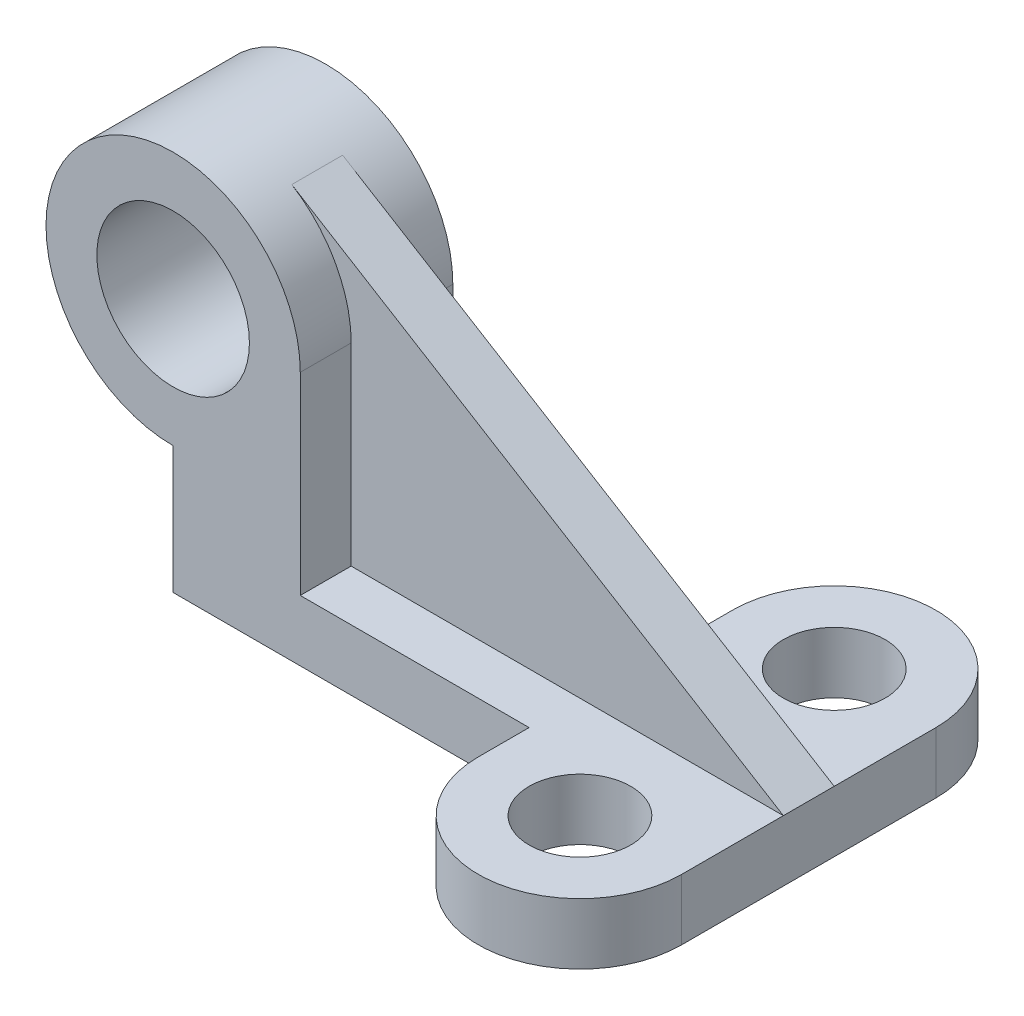
ISO-10303-21;
HEADER;
FILE_DESCRIPTION(('STEP AP214'),'2;1');
FILE_NAME('part.step','',(''),(''),'','','');
FILE_SCHEMA(('AUTOMOTIVE_DESIGN { 1 0 10303 214 1 1 1 1 }'));
ENDSEC;
DATA;
#1=APPLICATION_CONTEXT('core data for automotive mechanical design processes');
#2=APPLICATION_PROTOCOL_DEFINITION('international standard','automotive_design',2000,#1);
#3=PRODUCT_CONTEXT('',#1,'mechanical');
#4=PRODUCT('Part','Part','',(#3));
#5=PRODUCT_RELATED_PRODUCT_CATEGORY('part','',(#4));
#6=PRODUCT_DEFINITION_FORMATION('','',#4);
#7=PRODUCT_DEFINITION_CONTEXT('part definition',#1,'design');
#8=PRODUCT_DEFINITION('design','',#6,#7);
#9=PRODUCT_DEFINITION_SHAPE('','',#8);
#10=(LENGTH_UNIT() NAMED_UNIT(*) SI_UNIT(.MILLI.,.METRE.));
#11=(NAMED_UNIT(*) PLANE_ANGLE_UNIT() SI_UNIT($,.RADIAN.));
#12=(NAMED_UNIT(*) SI_UNIT($,.STERADIAN.) SOLID_ANGLE_UNIT());
#13=UNCERTAINTY_MEASURE_WITH_UNIT(LENGTH_MEASURE(1.E-05),#10,'distance_accuracy_value','');
#14=(GEOMETRIC_REPRESENTATION_CONTEXT(3) GLOBAL_UNCERTAINTY_ASSIGNED_CONTEXT((#13)) GLOBAL_UNIT_ASSIGNED_CONTEXT((#10,
#11,#12)) REPRESENTATION_CONTEXT('',''));
#15=CARTESIAN_POINT('',(0.,0.,0.));
#16=DIRECTION('',(0.,0.,1.));
#17=DIRECTION('',(1.,0.,0.));
#18=AXIS2_PLACEMENT_3D('',#15,#16,#17);
#19=CARTESIAN_POINT('',(0.,0.,0.));
#20=DIRECTION('',(0.,0.,1.));
#21=DIRECTION('',(1.,0.,0.));
#22=AXIS2_PLACEMENT_3D('',#19,#20,#21);
#23=PLANE('',#22);
#24=CARTESIAN_POINT('',(0.,0.,0.));
#25=DIRECTION('',(0.,0.,1.));
#26=DIRECTION('',(1.,0.,0.));
#27=AXIS2_PLACEMENT_3D('',#24,#25,#26);
#28=CIRCLE('',#27,15.);
#29=CARTESIAN_POINT('',(15.,0.,0.));
#30=VERTEX_POINT('',#29);
#31=EDGE_CURVE('E293',#30,#30,#28,.T.);
#32=ORIENTED_EDGE('',*,*,#31,.T.);
#33=EDGE_LOOP('',(#32));
#34=FACE_BOUND('',#33,.T.);
#35=DIRECTION('',(0.,1.,0.));
#36=VECTOR('',#35,1.);
#37=CARTESIAN_POINT('',(70.,-50.,0.));
#38=LINE('',#37,#36);
#39=CARTESIAN_POINT('',(70.,-50.,0.));
#40=VERTEX_POINT('',#39);
#41=CARTESIAN_POINT('',(70.,-38.,0.));
#42=VERTEX_POINT('',#41);
#43=EDGE_CURVE('E59',#40,#42,#38,.T.);
#44=ORIENTED_EDGE('',*,*,#43,.F.);
#45=DIRECTION('',(1.,0.,0.));
#46=VECTOR('',#45,1.);
#47=CARTESIAN_POINT('',(0.,-50.,0.));
#48=LINE('',#47,#46);
#49=CARTESIAN_POINT('',(0.,-50.,0.));
#50=VERTEX_POINT('',#49);
#51=EDGE_CURVE('E343',#50,#40,#48,.T.);
#52=ORIENTED_EDGE('',*,*,#51,.F.);
#53=DIRECTION('',(0.,-1.,0.));
#54=VECTOR('',#53,1.);
#55=CARTESIAN_POINT('',(0.,-25.,0.));
#56=LINE('',#55,#54);
#57=CARTESIAN_POINT('',(0.,-25.,0.));
#58=VERTEX_POINT('',#57);
#59=EDGE_CURVE('E352',#58,#50,#56,.T.);
#60=ORIENTED_EDGE('',*,*,#59,.F.);
#61=CARTESIAN_POINT('',(0.,0.,0.));
#62=DIRECTION('',(0.,0.,1.));
#63=DIRECTION('',(1.,0.,0.));
#64=AXIS2_PLACEMENT_3D('',#61,#62,#63);
#65=CIRCLE('',#64,25.);
#66=CARTESIAN_POINT('',(25.,0.,0.));
#67=VERTEX_POINT('',#66);
#68=EDGE_CURVE('E49',#67,#58,#65,.T.);
#69=ORIENTED_EDGE('',*,*,#68,.F.);
#70=DIRECTION('',(0.,1.,0.));
#71=VECTOR('',#70,1.);
#72=CARTESIAN_POINT('',(25.,-38.,0.));
#73=LINE('',#72,#71);
#74=CARTESIAN_POINT('',(25.,-38.,0.));
#75=VERTEX_POINT('',#74);
#76=EDGE_CURVE('E333',#75,#67,#73,.T.);
#77=ORIENTED_EDGE('',*,*,#76,.F.);
#78=DIRECTION('',(-1.,0.,0.));
#79=VECTOR('',#78,1.);
#80=CARTESIAN_POINT('',(80.,-38.,0.));
#81=LINE('',#80,#79);
#82=EDGE_CURVE('E340',#42,#75,#81,.T.);
#83=ORIENTED_EDGE('',*,*,#82,.F.);
#84=EDGE_LOOP('',(#44,#52,#60,#69,#77,#83));
#85=FACE_BOUND('',#84,.T.);
#86=ADVANCED_FACE('F39',(#34,#85),#23,.F.);
#87=CARTESIAN_POINT('',(0.,0.,30.));
#88=DIRECTION('',(0.,0.,1.));
#89=DIRECTION('',(1.,0.,0.));
#90=AXIS2_PLACEMENT_3D('',#87,#88,#89);
#91=PLANE('',#90);
#92=CARTESIAN_POINT('',(0.,0.,30.));
#93=DIRECTION('',(0.,0.,1.));
#94=DIRECTION('',(1.,0.,0.));
#95=AXIS2_PLACEMENT_3D('',#92,#93,#94);
#96=CIRCLE('',#95,15.);
#97=CARTESIAN_POINT('',(15.,0.,30.));
#98=VERTEX_POINT('',#97);
#99=EDGE_CURVE('E298',#98,#98,#96,.T.);
#100=ORIENTED_EDGE('',*,*,#99,.F.);
#101=EDGE_LOOP('',(#100));
#102=FACE_BOUND('',#101,.T.);
#103=DIRECTION('',(1.,0.,0.));
#104=VECTOR('',#103,1.);
#105=CARTESIAN_POINT('',(0.,-50.,30.));
#106=LINE('',#105,#104);
#107=CARTESIAN_POINT('',(0.,-50.,30.));
#108=VERTEX_POINT('',#107);
#109=CARTESIAN_POINT('',(70.,-50.,30.));
#110=VERTEX_POINT('',#109);
#111=EDGE_CURVE('E346',#108,#110,#106,.T.);
#112=ORIENTED_EDGE('',*,*,#111,.T.);
#113=DIRECTION('',(0.,1.,0.));
#114=VECTOR('',#113,1.);
#115=CARTESIAN_POINT('',(70.,-50.,30.));
#116=LINE('',#115,#114);
#117=CARTESIAN_POINT('',(70.,-38.,30.));
#118=VERTEX_POINT('',#117);
#119=EDGE_CURVE('E196',#110,#118,#116,.T.);
#120=ORIENTED_EDGE('',*,*,#119,.T.);
#121=DIRECTION('',(-1.,0.,0.));
#122=VECTOR('',#121,1.);
#123=CARTESIAN_POINT('',(80.,-38.,30.));
#124=LINE('',#123,#122);
#125=CARTESIAN_POINT('',(25.,-38.,30.));
#126=VERTEX_POINT('',#125);
#127=EDGE_CURVE('E353',#118,#126,#124,.T.);
#128=ORIENTED_EDGE('',*,*,#127,.T.);
#129=DIRECTION('',(0.,1.,0.));
#130=VECTOR('',#129,1.);
#131=CARTESIAN_POINT('',(25.,-38.,30.));
#132=LINE('',#131,#130);
#133=CARTESIAN_POINT('',(25.,0.,30.));
#134=VERTEX_POINT('',#133);
#135=EDGE_CURVE('E324',#126,#134,#132,.T.);
#136=ORIENTED_EDGE('',*,*,#135,.T.);
#137=CARTESIAN_POINT('',(0.,0.,30.));
#138=DIRECTION('',(0.,0.,1.));
#139=DIRECTION('',(1.,0.,0.));
#140=AXIS2_PLACEMENT_3D('',#137,#138,#139);
#141=CIRCLE('',#140,25.);
#142=CARTESIAN_POINT('',(0.,-25.,30.));
#143=VERTEX_POINT('',#142);
#144=EDGE_CURVE('E11',#134,#143,#141,.T.);
#145=ORIENTED_EDGE('',*,*,#144,.T.);
#146=DIRECTION('',(0.,-1.,0.));
#147=VECTOR('',#146,1.);
#148=CARTESIAN_POINT('',(0.,-25.,30.));
#149=LINE('',#148,#147);
#150=EDGE_CURVE('E344',#143,#108,#149,.T.);
#151=ORIENTED_EDGE('',*,*,#150,.T.);
#152=EDGE_LOOP('',(#112,#120,#128,#136,#145,#151));
#153=FACE_BOUND('',#152,.T.);
#154=ADVANCED_FACE('F282',(#102,#153),#91,.T.);
#155=CARTESIAN_POINT('',(0.,0.,30.));
#156=DIRECTION('',(0.,0.,-1.));
#157=DIRECTION('',(-1.,0.,0.));
#158=AXIS2_PLACEMENT_3D('',#155,#156,#157);
#159=CYLINDRICAL_SURFACE('',#158,25.);
#160=CARTESIAN_POINT('',(13.33493929526,21.1466166086145,20.));
#161=CARTESIAN_POINT('',(18.7792232306046,17.713481316683,20.));
#162=CARTESIAN_POINT('',(21.890334423913,12.0753160956246,20.));
#163=CARTESIAN_POINT('',(25.,6.43977071944921,20.));
#164=CARTESIAN_POINT('',(25.,0.,20.));
#165=B_SPLINE_CURVE_WITH_KNOTS('',2,(#160,#161,#162,#163,#164),.UNSPECIFIED.,.F.,.F.,(3,2,3),
(0.,0.5,1.),.UNSPECIFIED.);
#166=CARTESIAN_POINT('',(13.3325159789368,21.1428810416085,20.));
#167=VERTEX_POINT('',#166);
#168=CARTESIAN_POINT('',(25.,0.,20.));
#169=VERTEX_POINT('',#168);
#170=EDGE_CURVE('E158',#167,#169,#165,.T.);
#171=ORIENTED_EDGE('',*,*,#170,.F.);
#172=DIRECTION('',(0.,0.,-1.));
#173=VECTOR('',#172,1.);
#174=CARTESIAN_POINT('',(13.3349392952599,21.1466166086146,30.));
#175=LINE('',#174,#173);
#176=CARTESIAN_POINT('',(13.333271356551,21.1440454639604,10.));
#177=VERTEX_POINT('',#176);
#178=EDGE_CURVE('E217',#177,#167,#175,.F.);
#179=ORIENTED_EDGE('',*,*,#178,.F.);
#180=CARTESIAN_POINT('',(0.,0.,10.));
#181=DIRECTION('',(0.,0.,-1.));
#182=DIRECTION('',(0.5333975718104,0.84586466434458,0.));
#183=AXIS2_PLACEMENT_3D('',#180,#181,#182);
#184=CIRCLE('',#183,25.);
#185=CARTESIAN_POINT('',(25.,0.,10.));
#186=VERTEX_POINT('',#185);
#187=EDGE_CURVE('E225',#177,#186,#184,.T.);
#188=ORIENTED_EDGE('',*,*,#187,.T.);
#189=DIRECTION('',(0.,0.,1.));
#190=VECTOR('',#189,1.);
#191=CARTESIAN_POINT('',(25.,0.,0.));
#192=LINE('',#191,#190);
#193=EDGE_CURVE('E303',#67,#186,#192,.T.);
#194=ORIENTED_EDGE('',*,*,#193,.F.);
#195=ORIENTED_EDGE('',*,*,#68,.T.);
#196=DIRECTION('',(0.,0.,1.));
#197=VECTOR('',#196,1.);
#198=CARTESIAN_POINT('',(0.,-25.,0.));
#199=LINE('',#198,#197);
#200=EDGE_CURVE('E302',#58,#143,#199,.T.);
#201=ORIENTED_EDGE('',*,*,#200,.T.);
#202=ORIENTED_EDGE('',*,*,#144,.F.);
#203=EDGE_CURVE('E42',#169,#134,#192,.T.);
#204=ORIENTED_EDGE('',*,*,#203,.F.);
#205=EDGE_LOOP('',(#171,#179,#188,#194,#195,#201,#202,#204));
#206=FACE_BOUND('',#205,.T.);
#207=ADVANCED_FACE('F41',(#206),#159,.T.);
#208=CARTESIAN_POINT('',(25.,-38.,0.));
#209=DIRECTION('',(1.,0.,0.));
#210=DIRECTION('',(0.,0.,-1.));
#211=AXIS2_PLACEMENT_3D('',#208,#209,#210);
#212=PLANE('',#211);
#213=DIRECTION('',(0.,0.,1.));
#214=VECTOR('',#213,1.);
#215=CARTESIAN_POINT('',(25.,-38.,0.));
#216=LINE('',#215,#214);
#217=CARTESIAN_POINT('',(25.,-38.,20.));
#218=VERTEX_POINT('',#217);
#219=EDGE_CURVE('E329',#218,#126,#216,.T.);
#220=ORIENTED_EDGE('',*,*,#219,.F.);
#221=DIRECTION('',(0.,-1.,0.));
#222=VECTOR('',#221,1.);
#223=CARTESIAN_POINT('',(25.,0.,20.));
#224=LINE('',#223,#222);
#225=EDGE_CURVE('E211',#169,#218,#224,.T.);
#226=ORIENTED_EDGE('',*,*,#225,.F.);
#227=ORIENTED_EDGE('',*,*,#203,.T.);
#228=ORIENTED_EDGE('',*,*,#135,.F.);
#229=EDGE_LOOP('',(#220,#226,#227,#228));
#230=FACE_BOUND('',#229,.T.);
#231=ADVANCED_FACE('F271',(#230),#212,.T.);
#232=CARTESIAN_POINT('',(80.,-38.,0.));
#233=DIRECTION('',(0.,1.,0.));
#234=DIRECTION('',(-1.,0.,0.));
#235=AXIS2_PLACEMENT_3D('',#232,#233,#234);
#236=PLANE('',#235);
#237=CARTESIAN_POINT('',(90.,-38.,40.));
#238=DIRECTION('',(0.,1.,0.));
#239=DIRECTION('',(-1.,0.,0.));
#240=AXIS2_PLACEMENT_3D('',#237,#238,#239);
#241=CIRCLE('',#240,9.99999999999999);
#242=CARTESIAN_POINT('',(80.,-38.,40.));
#243=VERTEX_POINT('',#242);
#244=EDGE_CURVE('E183',#243,#243,#241,.T.);
#245=ORIENTED_EDGE('',*,*,#244,.F.);
#246=EDGE_LOOP('',(#245));
#247=FACE_BOUND('',#246,.T.);
#248=DIRECTION('',(0.,0.,1.));
#249=VECTOR('',#248,1.);
#250=CARTESIAN_POINT('',(110.,-38.,0.));
#251=LINE('',#250,#249);
#252=CARTESIAN_POINT('',(110.,-38.,20.));
#253=VERTEX_POINT('',#252);
#254=CARTESIAN_POINT('',(110.,-38.,40.));
#255=VERTEX_POINT('',#254);
#256=EDGE_CURVE('E160',#253,#255,#251,.T.);
#257=ORIENTED_EDGE('',*,*,#256,.F.);
#258=DIRECTION('',(1.,0.,0.));
#259=VECTOR('',#258,1.);
#260=CARTESIAN_POINT('',(25.,-38.,20.));
#261=LINE('',#260,#259);
#262=EDGE_CURVE('E210',#218,#253,#261,.T.);
#263=ORIENTED_EDGE('',*,*,#262,.F.);
#264=ORIENTED_EDGE('',*,*,#219,.T.);
#265=ORIENTED_EDGE('',*,*,#127,.F.);
#266=DIRECTION('',(0.,0.,1.));
#267=VECTOR('',#266,1.);
#268=CARTESIAN_POINT('',(70.,-38.,40.));
#269=LINE('',#268,#267);
#270=CARTESIAN_POINT('',(70.,-38.,40.));
#271=VERTEX_POINT('',#270);
#272=EDGE_CURVE('E68',#118,#271,#269,.T.);
#273=ORIENTED_EDGE('',*,*,#272,.T.);
#274=CARTESIAN_POINT('',(90.,-38.,40.));
#275=DIRECTION('',(0.,1.,0.));
#276=DIRECTION('',(1.,0.,0.));
#277=AXIS2_PLACEMENT_3D('',#274,#275,#276);
#278=CIRCLE('',#277,20.);
#279=EDGE_CURVE('E198',#271,#255,#278,.T.);
#280=ORIENTED_EDGE('',*,*,#279,.T.);
#281=EDGE_LOOP('',(#257,#263,#264,#265,#273,#280));
#282=FACE_BOUND('',#281,.T.);
#283=ADVANCED_FACE('F274',(#247,#282),#236,.T.);
#284=CARTESIAN_POINT('',(0.,0.,0.));
#285=DIRECTION('',(0.,0.,1.));
#286=DIRECTION('',(1.,0.,0.));
#287=AXIS2_PLACEMENT_3D('',#284,#285,#286);
#288=CYLINDRICAL_SURFACE('',#287,15.);
#289=ORIENTED_EDGE('',*,*,#31,.F.);
#290=EDGE_LOOP('',(#289));
#291=FACE_BOUND('',#290,.T.);
#292=ORIENTED_EDGE('',*,*,#99,.T.);
#293=EDGE_LOOP('',(#292));
#294=FACE_BOUND('',#293,.T.);
#295=ADVANCED_FACE('F267',(#291,#294),#288,.F.);
#296=DIRECTION('',(0.,-1.,0.));
#297=VECTOR('',#296,1.);
#298=CARTESIAN_POINT('',(25.,0.,10.));
#299=LINE('',#298,#297);
#300=CARTESIAN_POINT('',(25.,-38.,10.));
#301=VERTEX_POINT('',#300);
#302=EDGE_CURVE('E201',#186,#301,#299,.T.);
#303=ORIENTED_EDGE('',*,*,#302,.T.);
#304=EDGE_CURVE('E330',#75,#301,#216,.T.);
#305=ORIENTED_EDGE('',*,*,#304,.F.);
#306=ORIENTED_EDGE('',*,*,#76,.T.);
#307=ORIENTED_EDGE('',*,*,#193,.T.);
#308=EDGE_LOOP('',(#303,#305,#306,#307));
#309=FACE_BOUND('',#308,.T.);
#310=ADVANCED_FACE('F264',(#309),#212,.T.);
#311=CARTESIAN_POINT('',(90.,-38.,-10.));
#312=DIRECTION('',(0.,1.,0.));
#313=DIRECTION('',(-1.,0.,0.));
#314=AXIS2_PLACEMENT_3D('',#311,#312,#313);
#315=CIRCLE('',#314,9.99999999999999);
#316=CARTESIAN_POINT('',(80.,-38.,-10.));
#317=VERTEX_POINT('',#316);
#318=EDGE_CURVE('E177',#317,#317,#315,.T.);
#319=ORIENTED_EDGE('',*,*,#318,.F.);
#320=EDGE_LOOP('',(#319));
#321=FACE_BOUND('',#320,.T.);
#322=DIRECTION('',(1.,0.,0.));
#323=VECTOR('',#322,1.);
#324=CARTESIAN_POINT('',(25.,-38.,10.));
#325=LINE('',#324,#323);
#326=CARTESIAN_POINT('',(110.,-38.,10.));
#327=VERTEX_POINT('',#326);
#328=EDGE_CURVE('E215',#301,#327,#325,.T.);
#329=ORIENTED_EDGE('',*,*,#328,.T.);
#330=CARTESIAN_POINT('',(110.,-38.,-10.));
#331=VERTEX_POINT('',#330);
#332=EDGE_CURVE('E349',#331,#327,#251,.T.);
#333=ORIENTED_EDGE('',*,*,#332,.F.);
#334=CARTESIAN_POINT('',(90.,-38.,-10.));
#335=DIRECTION('',(0.,1.,0.));
#336=DIRECTION('',(-1.,0.,0.));
#337=AXIS2_PLACEMENT_3D('',#334,#335,#336);
#338=CIRCLE('',#337,20.);
#339=CARTESIAN_POINT('',(70.,-38.,-10.));
#340=VERTEX_POINT('',#339);
#341=EDGE_CURVE('E167',#331,#340,#338,.T.);
#342=ORIENTED_EDGE('',*,*,#341,.T.);
#343=DIRECTION('',(0.,0.,1.));
#344=VECTOR('',#343,1.);
#345=CARTESIAN_POINT('',(70.,-38.,-10.));
#346=LINE('',#345,#344);
#347=EDGE_CURVE('E171',#340,#42,#346,.T.);
#348=ORIENTED_EDGE('',*,*,#347,.T.);
#349=ORIENTED_EDGE('',*,*,#82,.T.);
#350=ORIENTED_EDGE('',*,*,#304,.T.);
#351=EDGE_LOOP('',(#329,#333,#342,#348,#349,#350));
#352=FACE_BOUND('',#351,.T.);
#353=ADVANCED_FACE('F268',(#321,#352),#236,.T.);
#354=CARTESIAN_POINT('',(0.,-50.,0.));
#355=DIRECTION('',(0.,-1.,0.));
#356=DIRECTION('',(0.,0.,-1.));
#357=AXIS2_PLACEMENT_3D('',#354,#355,#356);
#358=PLANE('',#357);
#359=CARTESIAN_POINT('',(90.,-50.,-10.));
#360=DIRECTION('',(0.,1.,0.));
#361=DIRECTION('',(-1.,0.,0.));
#362=AXIS2_PLACEMENT_3D('',#359,#360,#361);
#363=CIRCLE('',#362,9.99999999999999);
#364=CARTESIAN_POINT('',(80.,-50.,-10.));
#365=VERTEX_POINT('',#364);
#366=EDGE_CURVE('E185',#365,#365,#363,.T.);
#367=ORIENTED_EDGE('',*,*,#366,.T.);
#368=EDGE_LOOP('',(#367));
#369=FACE_BOUND('',#368,.T.);
#370=CARTESIAN_POINT('',(90.,-50.,40.));
#371=DIRECTION('',(0.,1.,0.));
#372=DIRECTION('',(-1.,0.,0.));
#373=AXIS2_PLACEMENT_3D('',#370,#371,#372);
#374=CIRCLE('',#373,9.99999999999999);
#375=CARTESIAN_POINT('',(80.,-50.,40.));
#376=VERTEX_POINT('',#375);
#377=EDGE_CURVE('E190',#376,#376,#374,.T.);
#378=ORIENTED_EDGE('',*,*,#377,.T.);
#379=EDGE_LOOP('',(#378));
#380=FACE_BOUND('',#379,.T.);
#381=ORIENTED_EDGE('',*,*,#111,.F.);
#382=DIRECTION('',(0.,0.,1.));
#383=VECTOR('',#382,1.);
#384=CARTESIAN_POINT('',(0.,-50.,0.));
#385=LINE('',#384,#383);
#386=EDGE_CURVE('E332',#50,#108,#385,.T.);
#387=ORIENTED_EDGE('',*,*,#386,.F.);
#388=ORIENTED_EDGE('',*,*,#51,.T.);
#389=DIRECTION('',(0.,0.,1.));
#390=VECTOR('',#389,1.);
#391=CARTESIAN_POINT('',(70.,-50.,-10.));
#392=LINE('',#391,#390);
#393=CARTESIAN_POINT('',(70.,-50.,-10.));
#394=VERTEX_POINT('',#393);
#395=EDGE_CURVE('E169',#394,#40,#392,.T.);
#396=ORIENTED_EDGE('',*,*,#395,.F.);
#397=CARTESIAN_POINT('',(90.,-50.,-10.));
#398=DIRECTION('',(0.,1.,0.));
#399=DIRECTION('',(-1.,0.,0.));
#400=AXIS2_PLACEMENT_3D('',#397,#398,#399);
#401=CIRCLE('',#400,20.);
#402=CARTESIAN_POINT('',(110.,-50.,-10.));
#403=VERTEX_POINT('',#402);
#404=EDGE_CURVE('E162',#403,#394,#401,.T.);
#405=ORIENTED_EDGE('',*,*,#404,.F.);
#406=DIRECTION('',(0.,0.,1.));
#407=VECTOR('',#406,1.);
#408=CARTESIAN_POINT('',(110.,-50.,0.));
#409=LINE('',#408,#407);
#410=CARTESIAN_POINT('',(110.,-50.,40.));
#411=VERTEX_POINT('',#410);
#412=EDGE_CURVE('E144',#403,#411,#409,.T.);
#413=ORIENTED_EDGE('',*,*,#412,.T.);
#414=CARTESIAN_POINT('',(90.,-50.,40.));
#415=DIRECTION('',(0.,1.,0.));
#416=DIRECTION('',(1.,0.,0.));
#417=AXIS2_PLACEMENT_3D('',#414,#415,#416);
#418=CIRCLE('',#417,20.);
#419=CARTESIAN_POINT('',(70.,-50.,40.));
#420=VERTEX_POINT('',#419);
#421=EDGE_CURVE('E194',#420,#411,#418,.T.);
#422=ORIENTED_EDGE('',*,*,#421,.F.);
#423=DIRECTION('',(0.,0.,1.));
#424=VECTOR('',#423,1.);
#425=CARTESIAN_POINT('',(70.,-50.,40.));
#426=LINE('',#425,#424);
#427=EDGE_CURVE('E195',#110,#420,#426,.T.);
#428=ORIENTED_EDGE('',*,*,#427,.F.);
#429=EDGE_LOOP('',(#381,#387,#388,#396,#405,#413,#422,#428));
#430=FACE_BOUND('',#429,.T.);
#431=ADVANCED_FACE('F173',(#369,#380,#430),#358,.T.);
#432=CARTESIAN_POINT('',(0.,-25.,0.));
#433=DIRECTION('',(-1.,0.,0.));
#434=DIRECTION('',(0.,-1.,0.));
#435=AXIS2_PLACEMENT_3D('',#432,#433,#434);
#436=PLANE('',#435);
#437=ORIENTED_EDGE('',*,*,#150,.F.);
#438=ORIENTED_EDGE('',*,*,#200,.F.);
#439=ORIENTED_EDGE('',*,*,#59,.T.);
#440=ORIENTED_EDGE('',*,*,#386,.T.);
#441=EDGE_LOOP('',(#437,#438,#439,#440));
#442=FACE_BOUND('',#441,.T.);
#443=ADVANCED_FACE('F262',(#442),#436,.T.);
#444=CARTESIAN_POINT('',(110.,-50.,0.));
#445=DIRECTION('',(1.,0.,0.));
#446=DIRECTION('',(0.,0.,-1.));
#447=AXIS2_PLACEMENT_3D('',#444,#445,#446);
#448=PLANE('',#447);
#449=ORIENTED_EDGE('',*,*,#256,.T.);
#450=DIRECTION('',(0.,1.,0.));
#451=VECTOR('',#450,1.);
#452=CARTESIAN_POINT('',(110.,-50.,40.));
#453=LINE('',#452,#451);
#454=EDGE_CURVE('E155',#411,#255,#453,.T.);
#455=ORIENTED_EDGE('',*,*,#454,.F.);
#456=ORIENTED_EDGE('',*,*,#412,.F.);
#457=DIRECTION('',(0.,1.,0.));
#458=VECTOR('',#457,1.);
#459=CARTESIAN_POINT('',(110.,-50.,-10.));
#460=LINE('',#459,#458);
#461=EDGE_CURVE('E149',#403,#331,#460,.T.);
#462=ORIENTED_EDGE('',*,*,#461,.T.);
#463=ORIENTED_EDGE('',*,*,#332,.T.);
#464=DIRECTION('',(0.,0.,-1.));
#465=VECTOR('',#464,1.);
#466=CARTESIAN_POINT('',(110.,-38.,20.));
#467=LINE('',#466,#465);
#468=EDGE_CURVE('E216',#253,#327,#467,.T.);
#469=ORIENTED_EDGE('',*,*,#468,.F.);
#470=EDGE_LOOP('',(#449,#455,#456,#462,#463,#469));
#471=FACE_BOUND('',#470,.T.);
#472=ADVANCED_FACE('F150',(#471),#448,.T.);
#473=CARTESIAN_POINT('',(-0.607605139838045,-0.345958865427095,20.));
#474=DIRECTION('',(0.,0.,-1.));
#475=DIRECTION('',(-1.,0.,0.));
#476=AXIS2_PLACEMENT_3D('',#473,#474,#475);
#477=PLANE('',#476);
#478=DIRECTION('',(-0.852993027350446,0.521922307715929,0.));
#479=VECTOR('',#478,1.);
#480=CARTESIAN_POINT('',(110.,-38.,20.));
#481=LINE('',#480,#479);
#482=EDGE_CURVE('E209',#253,#167,#481,.T.);
#483=ORIENTED_EDGE('',*,*,#482,.T.);
#484=ORIENTED_EDGE('',*,*,#170,.T.);
#485=ORIENTED_EDGE('',*,*,#225,.T.);
#486=ORIENTED_EDGE('',*,*,#262,.T.);
#487=EDGE_LOOP('',(#483,#484,#485,#486));
#488=FACE_BOUND('',#487,.T.);
#489=ADVANCED_FACE('F254',(#488),#477,.F.);
#490=CARTESIAN_POINT('',(-0.607605139838045,-0.345958865427095,10.));
#491=DIRECTION('',(0.,0.,-1.));
#492=DIRECTION('',(-1.,0.,0.));
#493=AXIS2_PLACEMENT_3D('',#490,#491,#492);
#494=PLANE('',#493);
#495=ORIENTED_EDGE('',*,*,#187,.F.);
#496=DIRECTION('',(-0.852993027350446,0.521922307715929,0.));
#497=VECTOR('',#496,1.);
#498=CARTESIAN_POINT('',(110.,-38.,10.));
#499=LINE('',#498,#497);
#500=EDGE_CURVE('E214',#327,#177,#499,.T.);
#501=ORIENTED_EDGE('',*,*,#500,.F.);
#502=ORIENTED_EDGE('',*,*,#328,.F.);
#503=ORIENTED_EDGE('',*,*,#302,.F.);
#504=EDGE_LOOP('',(#495,#501,#502,#503));
#505=FACE_BOUND('',#504,.T.);
#506=ADVANCED_FACE('F244',(#505),#494,.T.);
#507=CARTESIAN_POINT('',(110.,-38.,20.));
#508=DIRECTION('',(-0.521922307715929,-0.852993027350446,0.));
#509=DIRECTION('',(0.852993027350446,-0.521922307715929,0.));
#510=AXIS2_PLACEMENT_3D('',#507,#508,#509);
#511=PLANE('',#510);
#512=ORIENTED_EDGE('',*,*,#500,.T.);
#513=ORIENTED_EDGE('',*,*,#178,.T.);
#514=ORIENTED_EDGE('',*,*,#482,.F.);
#515=ORIENTED_EDGE('',*,*,#468,.T.);
#516=EDGE_LOOP('',(#512,#513,#514,#515));
#517=FACE_BOUND('',#516,.T.);
#518=ADVANCED_FACE('F255',(#517),#511,.F.);
#519=CARTESIAN_POINT('',(90.,-50.,40.));
#520=DIRECTION('',(0.,1.,0.));
#521=DIRECTION('',(-1.,0.,0.));
#522=AXIS2_PLACEMENT_3D('',#519,#520,#521);
#523=CYLINDRICAL_SURFACE('',#522,20.);
#524=ORIENTED_EDGE('',*,*,#279,.F.);
#525=DIRECTION('',(0.,1.,0.));
#526=VECTOR('',#525,1.);
#527=CARTESIAN_POINT('',(70.,-50.,40.));
#528=LINE('',#527,#526);
#529=EDGE_CURVE('E204',#420,#271,#528,.T.);
#530=ORIENTED_EDGE('',*,*,#529,.F.);
#531=ORIENTED_EDGE('',*,*,#421,.T.);
#532=ORIENTED_EDGE('',*,*,#454,.T.);
#533=EDGE_LOOP('',(#524,#530,#531,#532));
#534=FACE_BOUND('',#533,.T.);
#535=ADVANCED_FACE('F257',(#534),#523,.T.);
#536=CARTESIAN_POINT('',(70.,-50.,40.));
#537=DIRECTION('',(-1.,0.,0.));
#538=DIRECTION('',(0.,-1.,0.));
#539=AXIS2_PLACEMENT_3D('',#536,#537,#538);
#540=PLANE('',#539);
#541=ORIENTED_EDGE('',*,*,#272,.F.);
#542=ORIENTED_EDGE('',*,*,#119,.F.);
#543=ORIENTED_EDGE('',*,*,#427,.T.);
#544=ORIENTED_EDGE('',*,*,#529,.T.);
#545=EDGE_LOOP('',(#541,#542,#543,#544));
#546=FACE_BOUND('',#545,.T.);
#547=ADVANCED_FACE('F390',(#546),#540,.T.);
#548=CARTESIAN_POINT('',(90.,-50.,40.));
#549=DIRECTION('',(0.,1.,0.));
#550=DIRECTION('',(-1.,0.,0.));
#551=AXIS2_PLACEMENT_3D('',#548,#549,#550);
#552=CYLINDRICAL_SURFACE('',#551,9.99999999999999);
#553=ORIENTED_EDGE('',*,*,#377,.F.);
#554=EDGE_LOOP('',(#553));
#555=FACE_BOUND('',#554,.T.);
#556=ORIENTED_EDGE('',*,*,#244,.T.);
#557=EDGE_LOOP('',(#556));
#558=FACE_BOUND('',#557,.T.);
#559=ADVANCED_FACE('F386',(#555,#558),#552,.F.);
#560=CARTESIAN_POINT('',(70.,-50.,-10.));
#561=DIRECTION('',(-1.,0.,0.));
#562=DIRECTION('',(0.,0.,1.));
#563=AXIS2_PLACEMENT_3D('',#560,#561,#562);
#564=PLANE('',#563);
#565=ORIENTED_EDGE('',*,*,#347,.F.);
#566=DIRECTION('',(0.,1.,0.));
#567=VECTOR('',#566,1.);
#568=CARTESIAN_POINT('',(70.,-50.,-10.));
#569=LINE('',#568,#567);
#570=EDGE_CURVE('E170',#394,#340,#569,.T.);
#571=ORIENTED_EDGE('',*,*,#570,.F.);
#572=ORIENTED_EDGE('',*,*,#395,.T.);
#573=ORIENTED_EDGE('',*,*,#43,.T.);
#574=EDGE_LOOP('',(#565,#571,#572,#573));
#575=FACE_BOUND('',#574,.T.);
#576=ADVANCED_FACE('F379',(#575),#564,.T.);
#577=CARTESIAN_POINT('',(90.,-50.,-10.));
#578=DIRECTION('',(0.,1.,0.));
#579=DIRECTION('',(-1.,0.,0.));
#580=AXIS2_PLACEMENT_3D('',#577,#578,#579);
#581=CYLINDRICAL_SURFACE('',#580,20.);
#582=ORIENTED_EDGE('',*,*,#341,.F.);
#583=ORIENTED_EDGE('',*,*,#461,.F.);
#584=ORIENTED_EDGE('',*,*,#404,.T.);
#585=ORIENTED_EDGE('',*,*,#570,.T.);
#586=EDGE_LOOP('',(#582,#583,#584,#585));
#587=FACE_BOUND('',#586,.T.);
#588=ADVANCED_FACE('F165',(#587),#581,.T.);
#589=CARTESIAN_POINT('',(90.,-50.,-10.));
#590=DIRECTION('',(0.,1.,0.));
#591=DIRECTION('',(-1.,0.,0.));
#592=AXIS2_PLACEMENT_3D('',#589,#590,#591);
#593=CYLINDRICAL_SURFACE('',#592,9.99999999999999);
#594=ORIENTED_EDGE('',*,*,#366,.F.);
#595=EDGE_LOOP('',(#594));
#596=FACE_BOUND('',#595,.T.);
#597=ORIENTED_EDGE('',*,*,#318,.T.);
#598=EDGE_LOOP('',(#597));
#599=FACE_BOUND('',#598,.T.);
#600=ADVANCED_FACE('F399',(#596,#599),#593,.F.);
#601=CLOSED_SHELL('',(#86,#154,#207,#231,#283,#295,#310,#353,#431,#443,#472,#489,#506,#518,#535,
#547,#559,#576,#588,#600));
#602=MANIFOLD_SOLID_BREP('B2',#601);
#603=ADVANCED_BREP_SHAPE_REPRESENTATION('',(#18,#602),#14);
#604=SHAPE_DEFINITION_REPRESENTATION(#9,#603);
ENDSEC;
END-ISO-10303-21;
